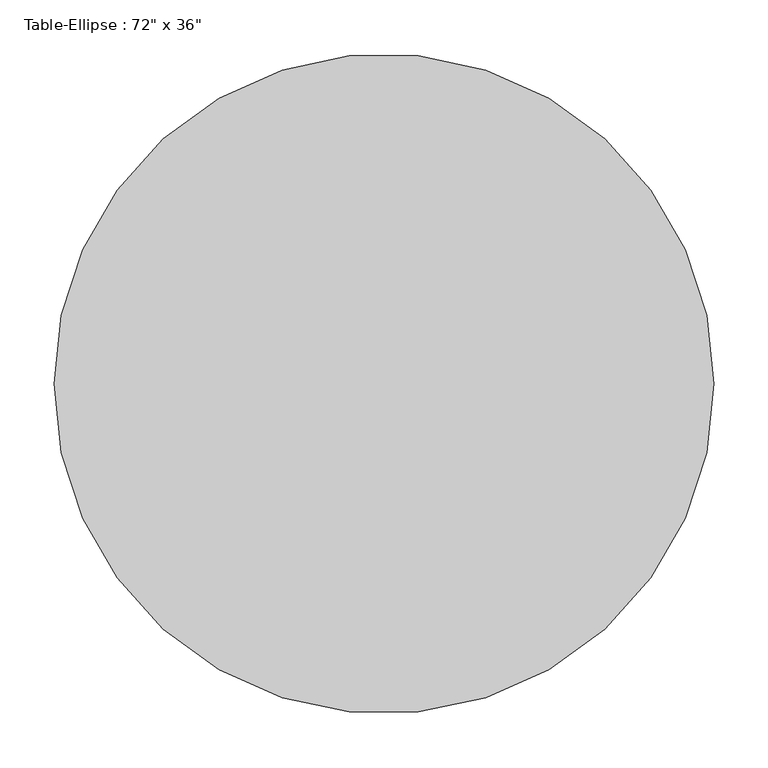
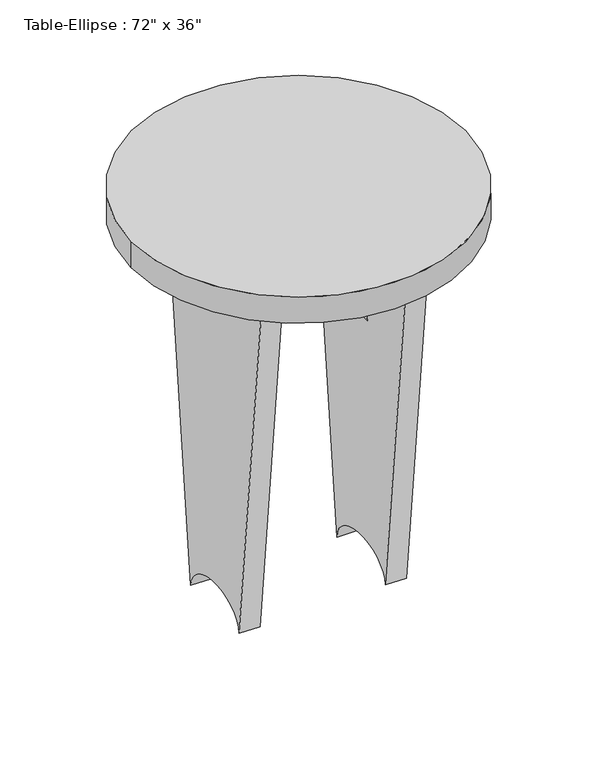
"""IFC4 building model written with IfcOpenShell, lengths in millimetres: furniture geometry."""

from ifc_helpers import new_model, si_unit, point, frame, origin, place, context, project, spatial, circle_curve, ellipse_curve, trimmed, source, transform, mapped, element, save
from ifc_brep_helpers import plane_surface, extruded_surface, advanced_brep


def furniture_f0d1c541(model_context):
    return source(origin(), model_context, "Body", "AdvancedBrep", [
        advanced_brep(
        [(-114.3, 19.05, 711.2), (114.3, 19.05, 711.2), (114.3, 19.05, 474.1333333), (-114.3, 19.05, 474.1333333), (-114.3, -19.05, 711.2), (-114.3, -19.05, 474.1333333), (114.3, -19.05, 474.1333333), (114.3, -19.05, 711.2)],
        [
            (0, 1),
            (1, 2),
            (2, 3, ellipse_curve(frame((0.0, 19.05, 474.1333333), z_axis=(0.0, -1.0, 0.0), x_axis=(1.0, 0.0, 0.0)), 114.3, 101.6)),
            (3, 0),
            (4, 5),
            (5, 6, ellipse_curve(frame((0.0, -19.05, 474.1333333), z_axis=(0.0, 1.0, 0.0), x_axis=(1.0, 0.0, 0.0)), 114.3, 101.6)),
            (6, 7),
            (7, 4),
            (0, 4),
            (7, 1),
            (6, 2),
            (5, 3),
        ],
        [
            plane_surface(frame((-114.3, 19.05, 711.2), z_axis=(0.0, 1.0, 0.0), x_axis=(1.0, 0.0, 0.0))),
            plane_surface(frame((-114.3, -19.05, 711.2), z_axis=(0.0, -1.0, 0.0), x_axis=(-1.0, 0.0, 0.0))),
            plane_surface(frame((-114.3, 19.05, 711.2), z_axis=(0.0, 0.0, 1.0), x_axis=(0.0, -1.0, 0.0))),
            plane_surface(frame((114.3, 19.05, 711.2), z_axis=(1.0, 0.0, 0.0), x_axis=(0.0, -1.0, 0.0))),
            extruded_surface(trimmed(ellipse_curve(frame((0.0, -57.15, 474.1333333), z_axis=(0.0, -1.0, 0.0), x_axis=(1.0, 0.0, 0.0)), 114.3, 101.6), [point((114.3, -57.15, 474.1333333))], [point((-114.3, -57.15, 474.1333333))], True, "CARTESIAN"), (0.0, 38.099999999999994, 0.0), 38.099999999999994),
            plane_surface(frame((-114.3, 19.05, 474.1333333), z_axis=(-1.0, 0.0, 0.0), x_axis=(0.0, -1.0, 0.0))),
        ],
        [
            (0, [[1, 2, 3, 4]]),
            (1, [[5, 6, 7, 8]]),
            (2, [[-1, 9, -8, 10]]),
            (3, [[-2, -10, -7, 11]]),
            (4, [[-3, -11, -6, 12]]),
            (5, [[-4, -12, -5, -9]]),
        ],
    ),
        advanced_brep(
        [(152.4, 152.4, 711.2), (152.4, -152.4, 711.2), (152.4, -76.2, 0.0), (152.4, 76.2, 0.0), (114.3, 152.4, 711.2), (114.3, 76.2, 0.0), (114.3, -76.2, 0.0), (114.3, -152.4, 711.2)],
        [
            (0, 1),
            (1, 2),
            (2, 3, ellipse_curve(frame((152.4, 0.0, 0.0), z_axis=(-1.0, 0.0, 0.0), x_axis=(0.0, 1.0, 0.0)), 76.2, 50.8)),
            (3, 0),
            (4, 5),
            (5, 6, ellipse_curve(frame((114.3, 0.0, 0.0), z_axis=(1.0, 0.0, 0.0), x_axis=(0.0, 1.0, 0.0)), 76.2, 50.8)),
            (6, 7),
            (7, 4),
            (0, 4),
            (7, 1),
            (6, 2),
            (5, 3),
        ],
        [
            plane_surface(frame((152.4, -152.4, 711.2), z_axis=(1.0, 0.0, 0.0), x_axis=(0.0, -1.0, 0.0))),
            plane_surface(frame((114.3, -152.4, 711.2), z_axis=(-1.0, 0.0, 0.0), x_axis=(0.0, 1.0, 0.0))),
            plane_surface(frame((152.4, 152.4, 711.2), z_axis=(0.0, 0.0, 1.0), x_axis=(-1.0, 0.0, 0.0))),
            plane_surface(frame((152.4, -152.4, 711.2), z_axis=(0.0, -0.9943091539198088, -0.10653312363426691), x_axis=(-1.0, 0.0, 0.0))),
            extruded_surface(trimmed(ellipse_curve(frame((76.2, 0.0, 0.0), z_axis=(-1.0, 0.0, 0.0), x_axis=(0.0, 1.0, 0.0)), 76.2, 50.8), [point((76.2, -76.2, 0.0))], [point((76.2, 76.2, 0.0))], True, "CARTESIAN"), (38.099999999999994, 0.0, 0.0), 38.099999999999994),
            plane_surface(frame((152.4, 76.2, 0.0), z_axis=(0.0, 0.9943091539198101, -0.10653312363425556), x_axis=(-1.0, 0.0, 0.0))),
        ],
        [
            (0, [[1, 2, 3, 4]]),
            (1, [[5, 6, 7, 8]]),
            (2, [[-1, 9, -8, 10]]),
            (3, [[-2, -10, -7, 11]]),
            (4, [[-3, -11, -6, 12]]),
            (5, [[-4, -12, -5, -9]]),
        ],
    ),
        advanced_brep(
        [(-114.3, 152.4, 711.2), (-114.3, -152.4, 711.2), (-114.3, -76.2, 0.0), (-114.3, 76.2, 0.0), (-152.4, 152.4, 711.2), (-152.4, 76.2, 0.0), (-152.4, -76.2, 0.0), (-152.4, -152.4, 711.2)],
        [
            (0, 1),
            (1, 2),
            (2, 3, ellipse_curve(frame((-114.3, 0.0, 0.0), z_axis=(-1.0, 0.0, 0.0), x_axis=(0.0, 1.0, 0.0)), 76.2, 50.8)),
            (3, 0),
            (4, 5),
            (5, 6, ellipse_curve(frame((-152.4, 0.0, 0.0), z_axis=(1.0, 0.0, 0.0), x_axis=(0.0, 1.0, 0.0)), 76.2, 50.8)),
            (6, 7),
            (7, 4),
            (0, 4),
            (7, 1),
            (6, 2),
            (5, 3),
        ],
        [
            plane_surface(frame((-114.3, -152.4, 711.2), z_axis=(1.0, 0.0, 0.0), x_axis=(0.0, -1.0, 0.0))),
            plane_surface(frame((-152.4, -152.4, 711.2), z_axis=(-1.0, 0.0, 0.0), x_axis=(0.0, 1.0, 0.0))),
            plane_surface(frame((-114.3, 152.4, 711.2), z_axis=(0.0, 0.0, 1.0), x_axis=(-1.0, 0.0, 0.0))),
            plane_surface(frame((-114.3, -152.4, 711.2), z_axis=(0.0, -0.9943091539198087, -0.10653312363426883), x_axis=(-1.0, 0.0, 0.0))),
            extruded_surface(trimmed(ellipse_curve(frame((-190.5, 0.0, 0.0), z_axis=(-1.0, 0.0, 0.0), x_axis=(0.0, 1.0, 0.0)), 76.2, 50.8), [point((-190.5, -76.2, 0.0))], [point((-190.5, 76.2, 0.0))], True, "CARTESIAN"), (38.099999999999994, 0.0, 0.0), 38.099999999999994),
            plane_surface(frame((-114.3, 76.2, 0.0), z_axis=(0.0, 0.9943091539198097, -0.10653312363425964), x_axis=(-1.0, 0.0, 0.0))),
        ],
        [
            (0, [[1, 2, 3, 4]]),
            (1, [[5, 6, 7, 8]]),
            (2, [[-1, 9, -8, 10]]),
            (3, [[-2, -10, -7, 11]]),
            (4, [[-3, -11, -6, 12]]),
            (5, [[-4, -12, -5, -9]]),
        ],
    ),
        advanced_brep(
        [(-304.8, 0.0, 762.0), (304.8, 0.0, 762.0), (-304.8, 0.0, 711.2), (304.8, 0.0, 711.2)],
        [
            (0, 1, circle_curve(frame((0.0, 0.0, 762.0), z_axis=(0.0, 0.0, 1.0), x_axis=(1.0, 0.0, 0.0)), 304.8)),
            (1, 0, circle_curve(frame((0.0, 0.0, 762.0), z_axis=(0.0, 0.0, 1.0), x_axis=(1.0, 0.0, 0.0)), 304.8)),
            (2, 3, ellipse_curve(frame((0.0, 0.0, 711.2), z_axis=(0.0, 0.0, -1.0), x_axis=(1.0, 0.0, 0.0)), 304.8, 304.8)),
            (3, 2, ellipse_curve(frame((0.0, 0.0, 711.2), z_axis=(0.0, 0.0, -1.0), x_axis=(1.0, 0.0, 0.0)), 304.8, 304.8)),
            (0, 2),
            (3, 1),
        ],
        [
            plane_surface(frame((304.8, 0.0, 762.0), z_axis=(0.0, 0.0, 1.0), x_axis=(0.0, 1.0, 0.0))),
            plane_surface(frame((304.8, 0.0, 711.2), z_axis=(0.0, 0.0, -1.0), x_axis=(0.0, -1.0, 0.0))),
            extruded_surface(trimmed(ellipse_curve(frame((0.0, 0.0, 660.4), z_axis=(0.0, 0.0, 1.0), x_axis=(1.0, 0.0, 0.0)), 304.8, 304.8), [point((-304.8, 0.0, 660.4))], [point((304.8, 0.0, 660.4))], True, "CARTESIAN"), (0.0, 0.0, 50.80000000000007), 50.80000000000007),
            extruded_surface(trimmed(ellipse_curve(frame((0.0, 0.0, 660.4), z_axis=(0.0, 0.0, 1.0), x_axis=(1.0, 0.0, 0.0)), 304.8, 304.8), [point((304.8, 0.0, 660.4))], [point((-304.8, 0.0, 660.4))], True, "CARTESIAN"), (0.0, 0.0, 50.80000000000007), 50.80000000000007),
        ],
        [
            (0, [[1, 2]]),
            (1, [[3, 4]]),
            (2, [[-1, 5, -4, 6]]),
            (3, [[-2, -6, -3, -5]]),
        ],
    ),
    ])


if __name__ == "__main__":
    model = new_model("IFC4")
    model_context = context("Model", 3, world=origin())
    ifc_project = project(units=[si_unit("LENGTHUNIT", "METRE", prefix="MILLI")], contexts=[model_context])
    site = spatial("IfcSite", under=ifc_project)
    building = spatial("IfcBuilding", under=site)
    placement = place(None, origin())
    furniture_shape = furniture_f0d1c541(model_context)
    element("IfcFurniture", 1, ObjectType="Table-Ellipse : 72\" x 36\"", at=placement, inside=building, context=model_context, shape_type="MappedRepresentation", body=[
        mapped(furniture_shape, transform((0.0, 0.0, 0.0), x_axis=(1.0, 0.0, 0.0), y_axis=(0.0, 1.0, 0.0), z_axis=(0.0, 0.0, 1.0))),
    ])
    save(model, "model.ifc")

# Revit data of these elements
# Type "Table-Ellipse : 72\" x 36\""
#   Assembly Code = "E2020200"
#   Half Width = 1' - 0"
#   Half Length = 1' - 0"
#   Height = 2' - 6"
#   Length = 2' - 0"
#   Width = 2' - 0"
#   Base Material = Birch
#   Top Material = Laminate - Black
#   Default Elevation = 0
# Element 1 (IfcFurniture, "Table-Ellipse : 72\" x 36\"")
#   Materials on its faces: "Birch", "Laminate - Black"
# Materials
#   "Birch": class "Wood", colour RGB 224 178 126, transparency 0, Description = "Betula Alleghaniensis", Cost = 0
#   "Laminate - Black": colour RGB 0 0 0, transparency 0
